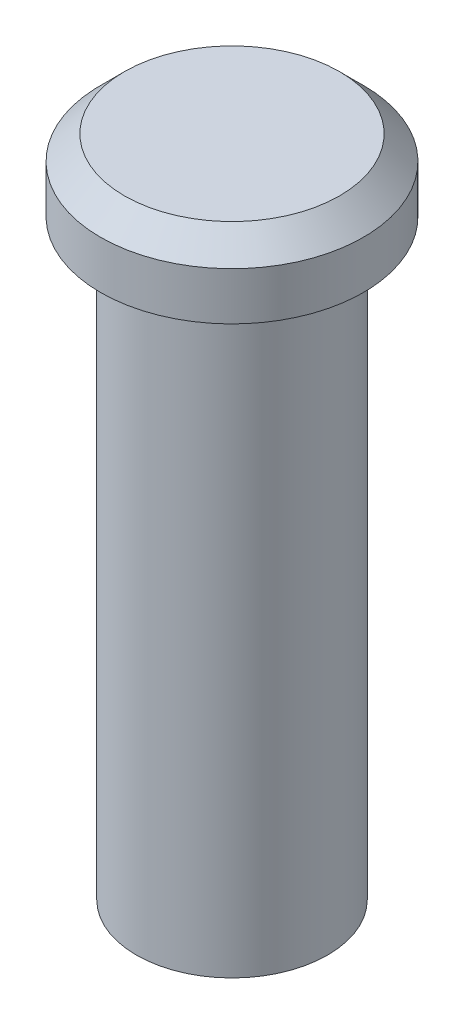
SolidWorks part; units mm, degrees
material "Plain Carbon Steel"
ref_plane "Front Plane" through (0, 0, 0) normal (0, 0, 1) x (1, 0, 0)
ref_plane "Top Plane" through (0, 0, 0) normal (0, 1, 0) x (1, 0, 0)
ref_plane "Right Plane" through (0, 0, 0) normal (1, 0, 0) x (0, 0, -1)
sketch "Shank Profile Ø8" plane through (0, 0, 0) normal (0, 1, 0) x (1, 0, 0)
  circle A0 centre (0, 0) radius 4
  dimension "D1" = 8
extrude "Shank Ø8" add sketch "Shank Profile Ø8" along normal blind 24.75
sketch "Head Profile Ø14" plane through (0, 24.75, 0) normal (0, 1, 0) x (1, 0, 0)
  circle A0 centre (0, 0) radius 5.5
  dimension "D1" = 11
extrude "Head Ø14" add sketch "Head Profile Ø14" along normal blind 3
chamfer "Head Chamfer 1x45°" distance 1 angle 45 1 edges at (0, 27.75, 5.5)
